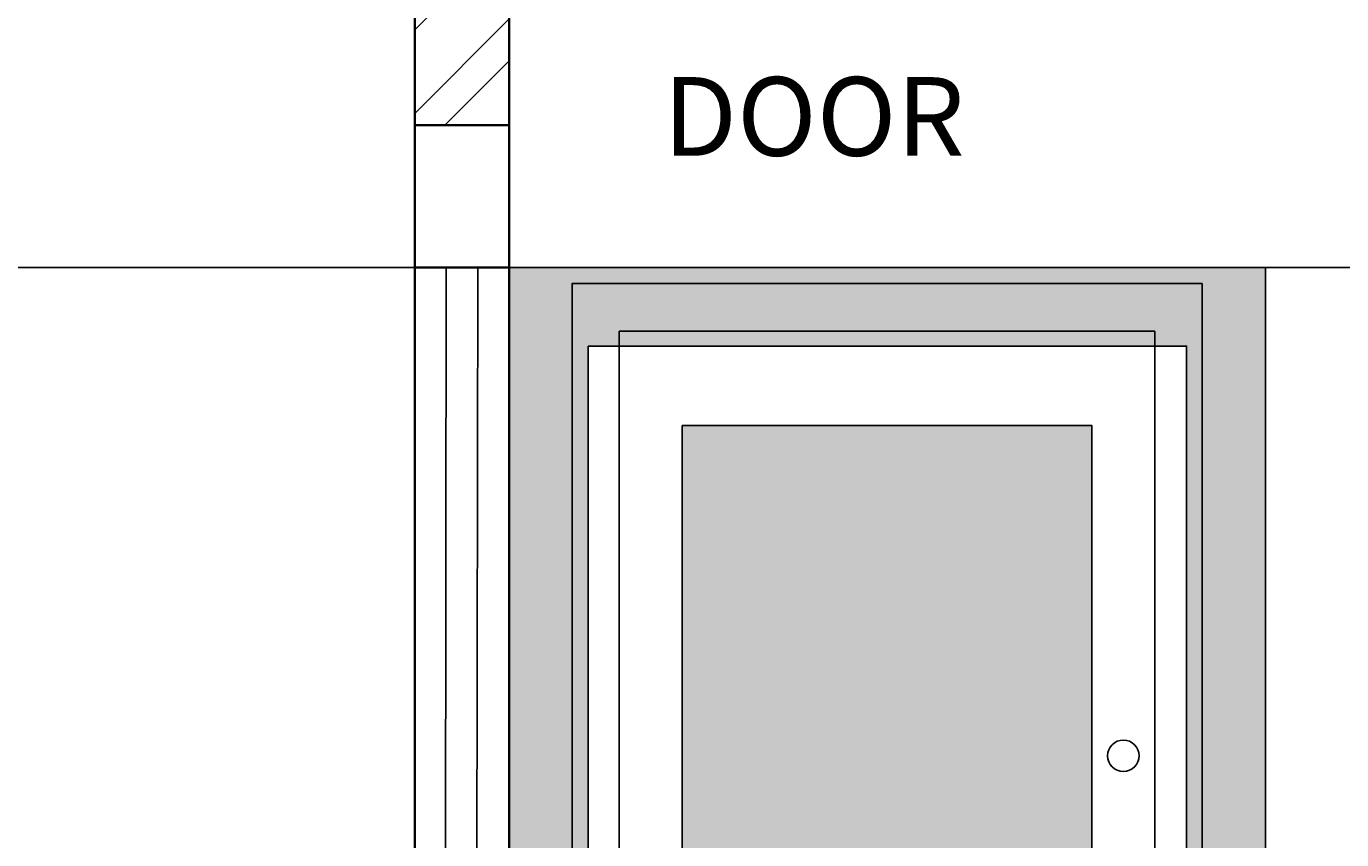
# Model space of a CAD drawing. Units: inches. Extents: x -301 to 715, y -607 to 364.
# Tile 24 of 141: x -66 to 18, y -422 to -370. Entities that reach past the tile are written whole.
import ezdxf

# ---------------------------------------------------------------- set-up
doc = ezdxf.new("R2010")
doc.units = ezdxf.units.IN
doc.header["$MEASUREMENT"] = 0
for name, color, linetype, lineweight in [('A-ANNO-DIMS', 2, 'Continuous', 18), ('A-ANNO-TEXT', 4, 'Continuous', 18), ('A-DOOR', 4, 'Continuous', 25), ('A-SECT', 1, 'Continuous', 35), ('A-SECT-PATT', 8, 'Continuous', 13)]:
    doc.layers.add(name, color=color, linetype=linetype, lineweight=lineweight)
doc.styles.get("Standard").update_dxf_attribs({"font": 'arial.ttf'})
doc.dimstyles.get("Standard").update_dxf_attribs({"dimtxt": 0.18, "dimasz": 0.18, "dimexe": 0.18, "dimexo": 0.0625, "dimgap": 0.09, "dimtad": 0, "dimtih": 1, "dimtoh": 1, "dimdec": 1, "dimzin": 0, "dimdsep": 46, "dimlunit": 4, "dimtxsty": 'Standard', "dimcen": 0.09, "dimclrd": 3, "dimclre": 4, "dimclrt": 6, "dimadec": 0, "dimazin": 0, "dimtfac": 1, "dimtdec": 1, "dimtofl": 0, "dimtmove": 0, "dimatfit": 3, "dimfxl": 1, "dimtfill": 2, "dimtfillclr": 51, "dimtolj": 1, "dimtzin": 0, "dimarcsym": 0})

# ---------------------------------------------------------------- blocks, each defined once
blk = doc.blocks.new('*U75')
blk.add_lwpolyline([(3.124, 0.013), (0.124, 0.013), (0.124, 72.013), (40.124, 72.013), (40.124, 0.013), (37.124, 0.013)])
for points in [[(37.124, 68.99), (37.124, 0.013), (3.124, 0.013), (3.124, 68.99)], [(33.124, 6.013), (33.124, 62.99), (7.124, 62.99), (7.124, 6.013)]]:
    blk.add_lwpolyline(points, close=True)
blk.add_circle((35.124, 42.013), 1)
blk = doc.blocks.new('*D176')
at = {"layer": 'A-ANNO-DIMS', "color": 4, "lineweight": -2, "transparency": 16777216}
for p, q in [((148.28, -324.477), (215.605, -324.477)), ((-15.22, -540.477), (215.605, -540.477))]:
    blk.add_line(p, q, dxfattribs=at)
at = {"layer": 'A-ANNO-DIMS', "color": 3, "lineweight": -2, "transparency": 16777216}
for p, q in [((215.425, -324.657), (215.425, -432.296)), ((215.425, -540.297), (215.425, -432.659))]:
    blk.add_line(p, q, dxfattribs=at)
at = {"layer": 'A-ANNO-DIMS', "color": 3, "transparency": 16777216}
for points in [[(215.395, -324.657), (215.455, -324.657), (215.425, -324.477)], [(215.395, -540.297), (215.455, -540.297), (215.425, -540.477)]]:
    blk.add_solid(points, dxfattribs=at)
at = {"layer": 'Defpoints', "color": 0, "transparency": 16777216}
for p in [(148.218, -324.477), (-15.282, -540.477), (215.425, -540.477)]:
    blk.add_point(p, dxfattribs=at)
at = {"layer": 'A-ANNO-DIMS', "color": 6, "transparency": 16777216, "insert": (215.425, -432.477), "char_height": 0.18, "attachment_point": 5, "bg_fill": 1, "box_fill_scale": 1.25, "bg_fill_color": 51, "bg_fill_transparency": 0}
blk.add_mtext('\\A1;18\'-0"', dxfattribs=at)
blk = doc.blocks.new('*D187')
at = {"layer": 'A-ANNO-DIMS', "color": 4, "lineweight": -2, "transparency": 16777216}
for p, q in [((139.674, -385.477), (-266.112, -385.477)), ((143.155, -439.477), (-266.112, -439.477))]:
    blk.add_line(p, q, dxfattribs=at)
at = {"layer": 'A-ANNO-DIMS', "color": 3, "lineweight": -2, "transparency": 16777216}
for p, q in [((-265.932, -385.657), (-265.932, -412.296)), ((-265.932, -439.297), (-265.932, -412.659))]:
    blk.add_line(p, q, dxfattribs=at)
at = {"layer": 'A-ANNO-DIMS', "color": 3, "transparency": 16777216}
for points in [[(-265.962, -385.657), (-265.902, -385.657), (-265.932, -385.477)], [(-265.962, -439.297), (-265.902, -439.297), (-265.932, -439.477)]]:
    blk.add_solid(points, dxfattribs=at)
at = {"layer": 'Defpoints', "color": 0, "transparency": 16777216}
for p in [(-265.932, -385.477), (139.737, -385.477), (143.218, -439.477)]:
    blk.add_point(p, dxfattribs=at)
at = {"layer": 'A-ANNO-DIMS', "color": 6, "transparency": 16777216, "insert": (-265.932, -412.477), "char_height": 0.18, "attachment_point": 5, "bg_fill": 1, "box_fill_scale": 1.25, "bg_fill_color": 51, "bg_fill_transparency": 0}
blk.add_mtext('\\A1;4\'-6"', dxfattribs=at)

msp = doc.modelspace()

# ---------------------------------------------------------------- hatches: boundary and pattern name
at = {"layer": 'A-SECT-PATT'}
h = msp.add_hatch(dxfattribs=at)
h.set_pattern_fill('ANSI32', color=256, scale=15)
h.set_pattern_definition([(45, (10.321, 33.8764), (-3.977476, 3.977476), []), (45, (12.973, 33.8764), (-3.977476, 3.977476), [])])
h.paths.add_polyline_path([(-35.282, -361.477), (-41.282, -361.477), (-41.282, -376.452), (-35.282, -376.452)])
h.paths.add_polyline_path([(143.218, -439.477), (134.255, -439.477), (134.255, -463.477), (143.218, -463.477)])
h = msp.add_hatch(color=256, dxfattribs=at)
h.dxf.hatch_style = 1
h.paths.add_polyline_path([(-138.282, -385.477), (-138.282, -433.477), (-87.981, -433.477), (-87.981, -385.477)])
h.paths.add_polyline_path([(-92.981, -390.477), (-92.981, -428.477), (-133.282, -428.477), (-133.282, -390.477)], flags=16)
h.paths.add_polyline_path([(-35.282, -385.477), (-35.282, -463.477), (12.718, -463.477), (12.718, -385.477)])
h.paths.add_polyline_path([(-30.282, -390.477), (7.718, -390.477), (7.718, -458.477), (-30.282, -458.477)], flags=16)
h.paths.add_polyline_path([(48.468, -385.477), (48.468, -433.477), (98.468, -433.477), (98.468, -385.477)])
h.paths.add_polyline_path([(93.468, -390.477), (93.468, -428.477), (53.468, -428.477), (53.468, -390.477)], flags=16)
h = msp.add_hatch(color=256, dxfattribs=at)
h.dxf.hatch_style = 1
h.paths.add_polyline_path([(-24.297, -452.509), (1.703, -452.509), (1.703, -395.532), (-24.297, -395.532)])

# ---------------------------------------------------------------- linework, layer by layer
at = {"layer": 'A-DOOR'}
for p, q in [((-39.282, -385.476), (-39.396, -463.476)), ((-37.282, -385.479), (-37.396, -463.479))]:
    msp.add_line(p, q, dxfattribs=at)
for points in [[(-35.282, -385.477), (12.718, -385.477), (12.718, -463.477), (-35.282, -463.477)], [(-30.282, -390.477), (7.718, -390.477), (7.718, -458.477), (-30.282, -458.477)]]:
    msp.add_lwpolyline(points, close=True, dxfattribs=at)
at = {"layer": 'A-SECT'}
for p, q in [((-41.282, -361.477), (-41.282, -481.477)), ((-35.282, -361.477), (-35.282, -463.477)), ((-41.282, -376.452), (-35.282, -376.452)), ((-41.282, -385.477), (-35.282, -385.477))]:
    msp.add_line(p, q, dxfattribs=at)

# ---------------------------------------------------------------- block references
at = {"layer": 'A-DOOR'}
msp.add_blockref('*U75', (-31.421, -458.522), dxfattribs=at)

# ---------------------------------------------------------------- texts
at = {"layer": 'A-ANNO-TEXT', "insert": (-25.515, -373.39), "char_height": 5, "attachment_point": 1}
msp.add_mtext_dynamic_manual_height_columns('DOOR', width=73.06001, gutter_width=1, heights=[0], dxfattribs=at)

# ---------------------------------------------------------------- dimensions: what is measured, and where the dimension line sits
at = {"layer": 'A-ANNO-DIMS'}
for base, p1, p2, picture, middle in [((215.425, -540.477), (148.218, -324.477), (-15.282, -540.477), '*D176', (215.425, -432.477)), ((-265.932, -385.477), (143.218, -439.477), (139.737, -385.477), '*D187', (-265.932, -412.477))]:
    dim = msp.add_linear_dim(base=base, p1=p1, p2=p2, angle=90, dimstyle='Standard', override={"dimdec": 1, "dimlfac": 1, "dimrnd": 0, "dimzin": 1, "dimdsep": 46, "dimlunit": 4, "dimfrac": 2}, dxfattribs=at)
    dim.commit()
    dim.dimension.update_dxf_attribs({"geometry": picture, "text_midpoint": middle})

doc.saveas('drawing.dxf')
